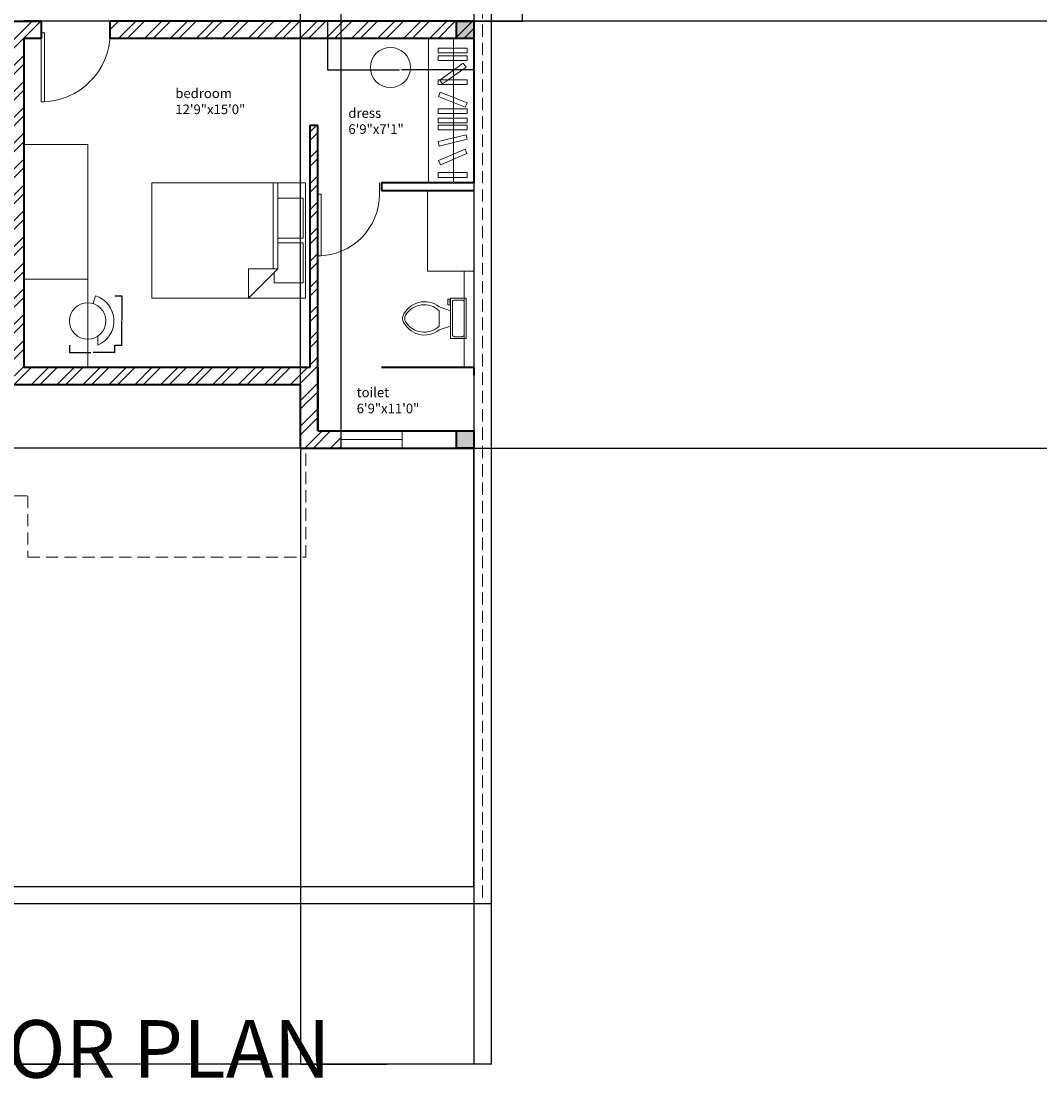
# Model space of a CAD drawing. Units: inches. Extents: x 19613 to 21413, y 12082 to 13202.
# Tile 2 of 9: x 19983 to 20513, y 12084 to 12634. Entities that reach past the tile are written whole.
import ezdxf

# ---------------------------------------------------------------- set-up
doc = ezdxf.new("R2010")
doc.units = ezdxf.units.IN
doc.linetypes.add('HIDDEN', pattern=[9.525, 6.35, -3.175])
for name, color, linetype, lineweight in [('A-ANNO-DIMS', 2, 'Continuous', 18), ('A-ANNO-TEXT', 7, 'Continuous', 30), ('A-AREA-IDEN', 7, 'Continuous', 18), ('A-COLS', 7, 'Continuous', 40), ('A-COLS-PATT', 6, 'Continuous', 13), ('A-DOOR', 3, 'Continuous', 18), ('A-FLOR-CASE', 9, 'Continuous', 18), ('A-FLOR-FIXT', 9, 'Continuous', 18), ('A-FLOR-HIDN', 8, 'HIDDEN', 13), ('A-FURN', 8, 'Continuous', 18), ('A-GLAZ', 4, 'Continuous', 18), ('A-WALL', 7, 'Continuous', 35), ('A-WALL-PATT', 252, 'Continuous', 13), ('C-PROP', 7, 'Continuous', 25), ('C-PROP-HIDN', 8, 'HIDDEN', 13)]:
    doc.layers.add(name, color=color, linetype=linetype, lineweight=lineweight)
doc.styles.get("Standard").update_dxf_attribs({"font": 'arial.ttf'})
doc.dimstyles.get("Standard").update_dxf_attribs({"dimtxt": 0.18, "dimasz": 0.18, "dimexe": 0.18, "dimexo": 0.0625, "dimgap": 0.09, "dimtad": 0, "dimtih": 1, "dimtoh": 1, "dimdec": 4, "dimzin": 0, "dimdsep": 46, "dimtxsty": 'Standard', "dimcen": 0.09, "dimadec": 0, "dimazin": 0, "dimtfac": 1, "dimtdec": 4, "dimtofl": 0, "dimtmove": 0, "dimatfit": 3, "dimfxl": 1, "dimtolj": 1, "dimtzin": 0, "dimarcsym": 0})

# ---------------------------------------------------------------- blocks, each defined once
blk = doc.blocks.new('Bed - Queen')
for p, q in [((0, -80.00003), (0, 0)), ((0, 0), (59.99999, 0)), ((59.99999, 0), (59.99999, -80.00003)), ((7.99999, -1.2), (28.79998, -1.2)), ((7.99999, -14.4), (7.99999, -1.2)), ((28.79998, -1.2), (28.79998, -14.4)), ((31.19999, -1.2), (51.99999, -1.2)), ((31.19999, -14.4), (31.19999, -1.2)), ((51.99999, -1.2), (51.99999, -16.4)), ((0, -14.4), (44.8, -14.4)), ((59.99999, -29.6), (44.8, -14.4)), ((44.8, -14.4), (44.8, -29.6)), ((51.99999, -16.4), (46.79936, -16.4)), ((44.8, -16.8), (0, -16.8)), ((44.8, -29.6), (59.99999, -29.6)), ((59.99999, -80.00003), (0, -80.00003))]:
    blk.add_line(p, q)
blk = doc.blocks.new('*U15')
for p, q in [((0, 0), (0, 6)), ((36, 0), (36, 6))]:
    blk.add_line(p, q)
blk.add_lwpolyline([(0, 0), (0, -36), (1.75, -36), (1.75, 0)], close=True)
blk.add_arc((0, 0), 36, 270, 0)
blk = doc.blocks.new('*U16')
for p, q in [((0, 0), (0, 6)), ((32, 0), (32, 6))]:
    blk.add_line(p, q)
blk.add_lwpolyline([(0, 0), (0, -32), (1.75, -32), (1.75, 0)], close=True)
blk.add_arc((0, 0), 32, 270, 0)
blk = doc.blocks.new('Toilet - top')
for p, q in [((9.5, -6), (9.5, -2)), ((-10, -8.5), (-8, -8.5)), ((-10, -9.5), (-10, -8.5)), ((-7, -9.5), (-10, -9.5)), ((-8, -8.5), (-8, -8)), ((-7, -8), (-7, -9.5)), ((-4, -8), (-6, -14)), ((4, -8), (6, -14)), ((4, -14), (-4, -14))]:
    blk.add_line(p, q)
blk.add_lwpolyline([(10.5, -8), (10.5, 0), (-10.5, 0), (-10.5, -8)], close=True)
for points in [[(-9.5, -2), (-9.5, -6)], [(8.5, -1), (-8.5, -1)], [(-8.5, -7), (8.5, -7)]]:
    blk.add_lwpolyline(points)
for centre, radius, start, end in [((-8.62, -1.88), 0.884, 81.8699, 188.1301), ((8.62, -1.88), 0.884, 351.8699, 98.1301), ((-8.62, -6.12), 0.884, 171.8699, 278.1301), ((8.62, -6.12), 0.884, 261.8699, 8.1301), ((3.52, -21.58), 12.17, 141.4691, 247.9714), ((4.2, -21.82), 11.33, 136.3677, 238.9468), ((-3.52, -21.58), 12.17, 292.0284, 38.5307), ((-4.2, -21.82), 11.33, 301.053, 43.6321), ((0, -27.88), 4, 245.7318, 294.2682), ((0, -29), 4, 254.8605, 285.1395)]:
    blk.add_arc(centre, radius, start, end)
blk = doc.blocks.new('COL-9x9')
for p, q in [((0, 9), (9, 9)), ((0, 0), (0, 9)), ((9, 9), (9, 0)), ((9, 0), (0, 0))]:
    blk.add_line(p, q)
blk = doc.blocks.new('CLOSET-STRAIGHT-RAIL')
for p, q in [((0, 75), (0, 0)), ((12.99, 75), (12.99, 0))]:
    blk.add_line(p, q)
for points in [[(5.04, 69.91), (20.08, 69.91), (20.08, 67.47), (5.04, 67.47)], [(5.04, 65.98), (20.08, 65.98), (20.08, 63.54), (5.04, 63.54)], [(5.8, 53.4), (18.07, 62.1), (19.48, 60.12), (7.21, 51.41)], [(5.04, 53.51), (20.08, 53.51), (20.08, 51.08), (5.04, 51.08)], [(6.02, 47.16), (20, 41.61), (19.1, 39.35), (5.12, 44.9)], [(5.04, 38.4), (20.08, 38.4), (20.08, 35.96), (5.04, 35.96)], [(5.04, 33.62), (20.08, 33.62), (20.08, 31.19), (5.04, 31.19)], [(5.04, 29.93), (20.08, 29.93), (20.08, 27.49), (5.04, 27.49)], [(4.97, 21.36), (19.58, 24.94), (20.16, 22.57), (5.55, 18.99)], [(5.22, 11.51), (19.01, 17.5), (19.98, 15.27), (6.19, 9.28)], [(5.04, 5.23), (20.08, 5.23), (20.08, 2.79), (5.04, 2.79)]]:
    blk.add_lwpolyline(points, close=True)
blk = doc.blocks.new('WINDOW-BATH')
for p, q in [((0, 9), (0, 0)), ((31.63, 9), (31.63, 0)), ((0, 4.5), (31.63, 4.5))]:
    blk.add_line(p, q)
blk = doc.blocks.new('DESK-CHAIR-ROUND-LARGE')
for p, q in [((13.49, 25.67), (12.27, 21.68)), ((14.77, 4.71), (14.81, 0))]:
    blk.add_line(p, q)
blk.add_circle((9.49, 12.6), 9.49)
blk.add_circle((9.49, 12.6), 9.49)
blk.add_arc((9.49, 12.6), 13.67, 292.8714, 73.0076)
blk = doc.blocks.new('BEDROOM-DESK-WIDE')
for p, q in [((33.29, 115.88), (0, 115.88)), ((33.29, 0), (33.29, 115.88)), ((33.29, 45.86), (0, 45.86)), ((0, 0), (0, 0)), ((0, 0), (33.29, 0))]:
    blk.add_line(p, q)
blk = doc.blocks.new('*D71')
at = {"layer": 'A-ANNO-DIMS', "color": 0, "lineweight": -2, "transparency": 16777216}
for p, q in [((20032, 12491.47), (20035.96, 12491.47)), ((20035.78, 12491.29), (20035.78, 12478.81)), ((20035.78, 12465.98), (20035.78, 12478.45)), ((20032, 12465.8), (20035.96, 12465.8))]:
    blk.add_line(p, q, dxfattribs=at)
at = {"layer": 'A-ANNO-DIMS', "color": 0, "transparency": 16777216}
for points in [[(20035.75, 12491.29), (20035.81, 12491.29), (20035.78, 12491.47)], [(20035.75, 12465.98), (20035.81, 12465.98), (20035.78, 12465.8)]]:
    blk.add_solid(points, dxfattribs=at)
at = {"layer": 'Defpoints', "color": 0, "transparency": 16777216}
for p in [(20031.93, 12491.47), (20035.78, 12491.47), (20031.93, 12465.8)]:
    blk.add_point(p, dxfattribs=at)
at = {"layer": 'A-ANNO-DIMS', "color": 0, "transparency": 16777216, "insert": (20035.78, 12478.63), "char_height": 0.18, "attachment_point": 5}
blk.add_mtext('\\A1;CHAIR 26 TYP.', dxfattribs=at)
blk = doc.blocks.new('*D72')
at = {"layer": 'A-ANNO-DIMS', "color": 0, "lineweight": -2, "transparency": 16777216}
for p, q in [((20008.49, 12465.73), (20008.49, 12461.76)), ((20031.93, 12465.73), (20031.93, 12461.76)), ((20008.67, 12461.94), (20019.68, 12461.94)), ((20031.75, 12461.94), (20020.74, 12461.94))]:
    blk.add_line(p, q, dxfattribs=at)
at = {"layer": 'A-ANNO-DIMS', "color": 0, "transparency": 16777216}
for points in [[(20008.67, 12461.97), (20008.67, 12461.91), (20008.49, 12461.94)], [(20031.75, 12461.97), (20031.75, 12461.91), (20031.93, 12461.94)]]:
    blk.add_solid(points, dxfattribs=at)
at = {"layer": 'Defpoints', "color": 0, "transparency": 16777216}
for p in [(20008.49, 12465.8), (20031.93, 12465.8), (20031.93, 12461.94)]:
    blk.add_point(p, dxfattribs=at)
at = {"layer": 'A-ANNO-DIMS', "color": 0, "transparency": 16777216, "insert": (20020.21, 12461.94), "char_height": 0.18, "attachment_point": 5}
blk.add_mtext('\\A1;23 TYP.', dxfattribs=at)
blk = doc.blocks.new('*D77')
at = {"layer": 'A-ANNO-DIMS', "color": 0, "lineweight": -2, "transparency": 16777216}
for p, q in [((20218.76, 12803.28), (20244.22, 12803.28)), ((20244.04, 12803.1), (20244.04, 12718.96)), ((20244.04, 12634.46), (20244.04, 12718.6)), ((20218.76, 12634.28), (20244.22, 12634.28))]:
    blk.add_line(p, q, dxfattribs=at)
at = {"layer": 'A-ANNO-DIMS', "color": 0, "transparency": 16777216}
for points in [[(20244.01, 12803.1), (20244.07, 12803.1), (20244.04, 12803.28)], [(20244.01, 12634.46), (20244.07, 12634.46), (20244.04, 12634.28)]]:
    blk.add_solid(points, dxfattribs=at)
at = {"layer": 'Defpoints', "color": 0, "transparency": 16777216}
for p in [(20218.69, 12803.28), (20244.04, 12803.28), (20218.69, 12634.28)]:
    blk.add_point(p, dxfattribs=at)
at = {"layer": 'A-ANNO-DIMS', "color": 0, "transparency": 16777216, "insert": (20244.04, 12718.78), "char_height": 0.18, "attachment_point": 5}
blk.add_mtext('\\A1;STAIR 169 TYP.', dxfattribs=at)
blk = doc.blocks.new('*D78')
at = {"layer": 'A-ANNO-DIMS', "color": 0, "lineweight": -2, "transparency": 16777216}
for p, q in [((20142.69, 12634.22), (20142.69, 12608.75)), ((20218.69, 12634.22), (20218.69, 12608.75)), ((20142.87, 12608.93), (20180.17, 12608.93)), ((20218.51, 12608.93), (20181.22, 12608.93))]:
    blk.add_line(p, q, dxfattribs=at)
at = {"layer": 'A-ANNO-DIMS', "color": 0, "transparency": 16777216}
for points in [[(20142.87, 12608.96), (20142.87, 12608.9), (20142.69, 12608.93)], [(20218.51, 12608.96), (20218.51, 12608.9), (20218.69, 12608.93)]]:
    blk.add_solid(points, dxfattribs=at)
at = {"layer": 'Defpoints', "color": 0, "transparency": 16777216}
for p in [(20142.69, 12634.28), (20218.69, 12634.28), (20218.69, 12608.93)]:
    blk.add_point(p, dxfattribs=at)
at = {"layer": 'A-ANNO-DIMS', "color": 0, "transparency": 16777216, "insert": (20180.69, 12608.93), "char_height": 0.18, "attachment_point": 5}
blk.add_mtext('\\A1;76 TYP.', dxfattribs=at)
blk = doc.blocks.new('*D83')
at = {"layer": 'A-ANNO-DIMS', "color": 0, "lineweight": -2, "transparency": 16777216}
for p, q in [((19696.69, 12175.22), (19696.69, 12091.85)), ((20227.69, 12175.22), (20227.69, 12091.85)), ((19696.87, 12092.03), (19961.92, 12092.03)), ((20227.51, 12092.03), (19962.47, 12092.03))]:
    blk.add_line(p, q, dxfattribs=at)
at = {"layer": 'A-ANNO-DIMS', "color": 0, "transparency": 16777216}
for points in [[(19696.87, 12092.06), (19696.87, 12092), (19696.69, 12092.03)], [(20227.51, 12092.06), (20227.51, 12092), (20227.69, 12092.03)]]:
    blk.add_solid(points, dxfattribs=at)
at = {"layer": 'Defpoints', "color": 0, "transparency": 16777216}
for p in [(19696.69, 12175.28), (20227.69, 12175.28), (20227.69, 12092.03)]:
    blk.add_point(p, dxfattribs=at)
at = {"layer": 'A-ANNO-DIMS', "color": 0, "transparency": 16777216, "insert": (19962.19, 12092.03), "char_height": 0.18, "attachment_point": 5}
blk.add_mtext('\\A1;531', dxfattribs=at)
blk = doc.blocks.new('*D87')
at = {"layer": 'A-ANNO-DIMS', "color": 0, "lineweight": -2, "transparency": 16777216}
for p, q in [((20218.76, 12982.28), (21412.86, 12982.28)), ((21412.68, 12982.1), (21412.68, 12697.46)), ((21412.68, 12412.46), (21412.68, 12697.1)), ((20218.76, 12412.28), (21412.86, 12412.28))]:
    blk.add_line(p, q, dxfattribs=at)
at = {"layer": 'A-ANNO-DIMS', "color": 0, "transparency": 16777216}
for points in [[(21412.65, 12982.1), (21412.71, 12982.1), (21412.68, 12982.28)], [(21412.65, 12412.46), (21412.71, 12412.46), (21412.68, 12412.28)]]:
    blk.add_solid(points, dxfattribs=at)
at = {"layer": 'Defpoints', "color": 0, "transparency": 16777216}
for p in [(20218.69, 12982.28), (21412.68, 12982.28), (20218.69, 12412.28)]:
    blk.add_point(p, dxfattribs=at)
at = {"layer": 'A-ANNO-DIMS', "color": 0, "transparency": 16777216, "insert": (21412.68, 12697.28), "char_height": 0.18, "attachment_point": 5}
blk.add_mtext('\\A1;570', dxfattribs=at)
blk = doc.blocks.new('*D89')
at = {"layer": 'A-ANNO-DIMS', "color": 0, "lineweight": -2, "transparency": 16777216}
for p, q in [((20807.37, 12808.28), (19613.26, 12808.28)), ((19613.44, 12808.1), (19613.44, 12721.46)), ((19613.44, 12634.46), (19613.44, 12721.1)), ((20807.37, 12634.28), (19613.26, 12634.28))]:
    blk.add_line(p, q, dxfattribs=at)
at = {"layer": 'A-ANNO-DIMS', "color": 0, "transparency": 16777216}
for points in [[(19613.41, 12808.1), (19613.47, 12808.1), (19613.44, 12808.28)], [(19613.41, 12634.46), (19613.47, 12634.46), (19613.44, 12634.28)]]:
    blk.add_solid(points, dxfattribs=at)
at = {"layer": 'Defpoints', "color": 0, "transparency": 16777216}
for p in [(19613.44, 12808.28), (20807.43, 12808.28), (20807.43, 12634.28)]:
    blk.add_point(p, dxfattribs=at)
at = {"layer": 'A-ANNO-DIMS', "color": 0, "transparency": 16777216, "insert": (19613.44, 12721.28), "char_height": 0.18, "attachment_point": 5}
blk.add_mtext('\\A1;174', dxfattribs=at)
blk = doc.blocks.new('*D92')
at = {"layer": 'A-ANNO-DIMS', "color": 0, "lineweight": -2, "transparency": 16777216}
for p, q in [((19903.69, 12445.22), (19903.69, 12091.85)), ((20128.69, 12445.22), (20128.69, 12091.85)), ((19903.87, 12092.03), (20015.9, 12092.03)), ((20128.51, 12092.03), (20016.48, 12092.03))]:
    blk.add_line(p, q, dxfattribs=at)
at = {"layer": 'A-ANNO-DIMS', "color": 0, "transparency": 16777216}
for points in [[(19903.87, 12092.06), (19903.87, 12092), (19903.69, 12092.03)], [(20128.51, 12092.06), (20128.51, 12092), (20128.69, 12092.03)]]:
    blk.add_solid(points, dxfattribs=at)
at = {"layer": 'Defpoints', "color": 0, "transparency": 16777216}
for p in [(19903.69, 12445.28), (20128.69, 12445.28), (20128.69, 12092.03)]:
    blk.add_point(p, dxfattribs=at)
at = {"layer": 'A-ANNO-DIMS', "color": 0, "transparency": 16777216, "insert": (20016.19, 12092.03), "char_height": 0.18, "attachment_point": 5}
blk.add_mtext('\\A1;225', dxfattribs=at)
blk = doc.blocks.new('*D93')
at = {"layer": 'A-ANNO-DIMS', "color": 0, "lineweight": -2, "transparency": 16777216}
for p, q in [((20128.69, 12412.22), (20128.69, 12091.85)), ((20218.69, 12412.22), (20218.69, 12091.85)), ((20128.87, 12092.03), (20173.48, 12092.03)), ((20218.51, 12092.03), (20173.91, 12092.03))]:
    blk.add_line(p, q, dxfattribs=at)
at = {"layer": 'A-ANNO-DIMS', "color": 0, "transparency": 16777216}
for points in [[(20128.87, 12092.06), (20128.87, 12092), (20128.69, 12092.03)], [(20218.51, 12092.06), (20218.51, 12092), (20218.69, 12092.03)]]:
    blk.add_solid(points, dxfattribs=at)
at = {"layer": 'Defpoints', "color": 0, "transparency": 16777216}
for p in [(20128.69, 12412.28), (20218.69, 12412.28), (20218.69, 12092.03)]:
    blk.add_point(p, dxfattribs=at)
at = {"layer": 'A-ANNO-DIMS', "color": 0, "transparency": 16777216, "insert": (20173.69, 12092.03), "char_height": 0.18, "attachment_point": 5}
blk.add_mtext('\\A1;90', dxfattribs=at)
blk = doc.blocks.new('*D97')
at = {"layer": 'A-ANNO-DIMS', "color": 0, "lineweight": -2, "transparency": 16777216}
for p, q in [((20128.63, 12445.28), (19613.26, 12445.28)), ((19613.44, 12445.1), (19613.44, 12428.96)), ((19613.44, 12412.46), (19613.44, 12428.6)), ((20128.63, 12412.28), (19613.26, 12412.28))]:
    blk.add_line(p, q, dxfattribs=at)
at = {"layer": 'A-ANNO-DIMS', "color": 0, "transparency": 16777216}
for points in [[(19613.41, 12445.1), (19613.47, 12445.1), (19613.44, 12445.28)], [(19613.41, 12412.46), (19613.47, 12412.46), (19613.44, 12412.28)]]:
    blk.add_solid(points, dxfattribs=at)
at = {"layer": 'Defpoints', "color": 0, "transparency": 16777216}
for p in [(19613.44, 12445.28), (20128.69, 12445.28), (20128.69, 12412.28)]:
    blk.add_point(p, dxfattribs=at)
at = {"layer": 'A-ANNO-DIMS', "color": 0, "transparency": 16777216, "insert": (19613.44, 12428.78), "char_height": 0.18, "attachment_point": 5}
blk.add_mtext('\\A1;33', dxfattribs=at)
blk = doc.blocks.new('*D107')
at = {"layer": 'A-ANNO-DIMS', "color": 0, "lineweight": -2, "transparency": 16777216}
for p, q in [((20128.69, 12412.34), (20128.69, 13201.71)), ((20128.87, 13201.53), (20138.81, 13201.53)), ((20149.67, 13201.53), (20139.74, 13201.53)), ((20149.85, 12412.34), (20149.85, 13201.71))]:
    blk.add_line(p, q, dxfattribs=at)
at = {"layer": 'A-ANNO-DIMS', "color": 0, "transparency": 16777216}
for points in [[(20128.87, 13201.56), (20128.87, 13201.5), (20128.69, 13201.53)], [(20149.67, 13201.56), (20149.67, 13201.5), (20149.85, 13201.53)]]:
    blk.add_solid(points, dxfattribs=at)
at = {"layer": 'Defpoints', "color": 0, "transparency": 16777216}
for p in [(20149.85, 13201.53), (20128.69, 12412.28), (20149.85, 12412.28)]:
    blk.add_point(p, dxfattribs=at)
at = {"layer": 'A-ANNO-DIMS', "color": 0, "transparency": 16777216, "insert": (20139.27, 13201.53), "char_height": 0.18, "attachment_point": 5}
blk.add_mtext('\\A1;21.154', dxfattribs=at)

msp = doc.modelspace()

# ---------------------------------------------------------------- hatches: boundary and pattern name
at = {"layer": 'A-COLS-PATT'}
h = msp.add_hatch(color=256, dxfattribs=at)
h.dxf.hatch_style = 1
h.paths.add_polyline_path([(19701.1937, 13118.279), (19696.6937, 13118.279), (19696.6937, 13113.779), (19701.1937, 13113.779)])
h.paths.add_polyline_path([(19714.6694, 12982.279), (19705.6937, 12982.279), (19705.6937, 12973.279), (19714.6694, 12973.279)])
h.paths.add_polyline_path([(19827.1183, 12982.279), (19818.1183, 12982.279), (19818.1183, 12973.279), (19827.1183, 12973.279)])
h.paths.add_polyline_path([(19982.6937, 12982.279), (19973.6937, 12982.279), (19973.6937, 12973.279), (19982.6937, 12973.279)])
h.paths.add_polyline_path([(19982.6937, 12817.279), (19973.6937, 12817.279), (19973.6937, 12808.279), (19982.6937, 12808.279)])
h.paths.add_polyline_path([(19795.361, 12817.279), (19786.361, 12817.279), (19786.361, 12808.279), (19795.361, 12808.279)])
h.paths.add_polyline_path([(19705.6937, 12817.279), (19702.0819, 12817.279), (19702.0819, 12808.279), (19705.6937, 12808.279)])
h.paths.add_polyline_path([(19711.0819, 12817.279), (19705.6937, 12817.279), (19705.6937, 12808.279), (19711.0819, 12808.279)])
h.paths.add_polyline_path([(19714.6136, 12634.279), (19705.6937, 12634.279), (19705.6937, 12625.279), (19714.6136, 12625.279)])
h.paths.add_polyline_path([(19705.6937, 12485.8897), (19701.1937, 12485.8897), (19701.1937, 12476.8897), (19705.6937, 12476.8897)])
h.paths.add_polyline_path([(19709.3479, 12485.8897), (19705.6937, 12485.8897), (19705.6937, 12476.8897), (19709.3479, 12476.8897)])
h.paths.add_polyline_path([(19701.1937, 12485.8897), (19700.3479, 12485.8897), (19700.3479, 12476.8897), (19701.1937, 12476.8897)])
h.paths.add_polyline_path([(20218.6937, 12421.279), (20209.6937, 12421.279), (20209.6937, 12412.279), (20218.6937, 12412.279)])
h.paths.add_polyline_path([(20218.6937, 12634.279), (20209.6937, 12634.279), (20209.6937, 12625.279), (20218.6937, 12625.279)])
h.paths.add_polyline_path([(20218.6937, 12808.279), (20209.6937, 12808.279), (20209.6937, 12803.279), (20218.6937, 12803.279)])
h.paths.add_polyline_path([(20218.6937, 12810.1878), (20209.6937, 12810.1878), (20209.6937, 12808.279), (20218.6937, 12808.279)])
h.paths.add_polyline_path([(20218.6937, 12803.279), (20209.6937, 12803.279), (20209.6937, 12801.1878), (20218.6937, 12801.1878)])
h.paths.add_polyline_path([(20218.6937, 12982.279), (20209.6937, 12982.279), (20209.6937, 12973.279), (20218.6937, 12973.279)])
h.paths.add_polyline_path([(20100.1214, 12982.279), (20080.8386, 12982.279), (20080.8386, 12973.279), (20091.6937, 12973.279), (20100.1214, 12973.279), (20100.1214, 12976.279)])
h.paths.add_polyline_path([(19851.5503, 12631.279), (19851.5503, 12634.279), (19828.8814, 12634.279), (19828.8814, 12625.279), (19851.5503, 12625.279)])
at = {"layer": 'A-WALL-PATT'}
h = msp.add_hatch(dxfattribs=at)
h.set_pattern_fill('ANSI32', color=256)
h.paths.add_polyline_path([(20223.1937, 13118.279), (20218.6937, 13118.279), (19701.1937, 13118.279), (19701.1937, 13113.779), (20223.1937, 13113.779)])
h.paths.add_polyline_path([(19849.7315, 12982.279), (19799.9854, 12982.279), (19799.9854, 12973.279), (19849.7315, 12973.279)])
h.paths.add_polyline_path([(19755.5378, 12982.279), (19705.6937, 12982.279), (19705.6937, 12973.279), (19755.5378, 12973.279)])
h.paths.add_polyline_path([(20000.1054, 12982.279), (19950.0534, 12982.279), (19950.0534, 12974.1171), (19950.0534, 12973.279), (20000.1054, 12973.279)])
h.paths.add_polyline_path([(20049.4797, 12982.279), (20030.7476, 12982.279), (20030.7476, 12973.279), (20049.4797, 12973.279)])
h.paths.add_polyline_path([(20100.1214, 12982.279), (20080.8386, 12982.279), (20080.8386, 12973.279), (20100.1214, 12973.279), (20100.1214, 12976.279)])
h.paths.add_polyline_path([(20218.6937, 12982.279), (20167.6937, 12982.279), (20140.1214, 12982.279), (20140.1214, 12976.279, -0.01769781), (20140.0212, 12973.45), (20167.6937, 12973.279), (20176.6937, 12973.279), (20218.6937, 12973.279)])
h.paths.add_polyline_path([(19851.5503, 12814.279), (19851.5503, 12817.279), (19793.6937, 12817.279), (19789.6937, 12817.279), (19705.6937, 12817.279), (19705.6937, 12808.279), (19851.5503, 12808.279)])
h.paths.add_polyline_path([(19982.6937, 12973.279), (19973.6937, 12973.279), (19973.6937, 12817.279), (19887.5503, 12817.279), (19887.5503, 12808.279), (19973.6937, 12808.279), (19982.6937, 12808.279)])
h.paths.add_polyline_path([(20058.6937, 12850.5529), (19982.6937, 12850.5529), (19982.6937, 12846.5529), (20058.6937, 12846.5529)])
h.paths.add_polyline_path([(20095.6937, 12973.279), (20091.6937, 12973.279), (20091.6937, 12850.5529), (20087.6937, 12850.5529), (20087.6937, 12846.5529), (20095.6937, 12846.5529)])
h.paths.add_polyline_path([(20218.6937, 12808.279), (20140.8605, 12808.279), (20126.9413, 12808.279), (20126.9413, 12803.279), (20140.8605, 12803.279), (20218.6937, 12803.279)])
h.paths.add_polyline_path([(19738.3931, 12634.279), (19705.6937, 12634.279), (19705.6937, 12625.279), (19738.3931, 12625.279)])
h.paths.add_polyline_path([(19912.6937, 12634.279), (19903.6937, 12634.279), (19891.5503, 12634.279), (19891.5503, 12625.279), (19903.6937, 12625.279), (19903.6937, 12445.279), (19975.6937, 12445.279), (20128.6937, 12445.279), (20128.6937, 12412.279), (20149.8479, 12412.279), (20149.8479, 12421.279), (20137.6937, 12421.279), (20137.6937, 12454.279), (20137.6937, 12580.2801), (20133.6937, 12580.2801), (20133.6937, 12454.279), (19984.6937, 12454.279), (19984.6937, 12625.279), (19993.6937, 12625.279), (19993.6937, 12634.279), (19984.6937, 12634.279), (19975.6937, 12634.279), (19975.6937, 12454.279), (19912.6937, 12454.279)])
h.paths.add_polyline_path([(20218.6937, 12634.279), (20137.6937, 12634.279), (20029.6937, 12634.279), (20029.6937, 12625.279), (20137.6937, 12625.279), (20218.6937, 12625.279)])
h.paths.add_polyline_path([(21014.4339, 12634.279), (21005.4339, 12634.279), (20993.2905, 12634.279), (20993.2905, 12625.279), (21005.4339, 12625.279), (21005.4339, 12445.279), (21077.4339, 12445.279), (21230.4339, 12445.279), (21230.4339, 12412.279), (21251.5881, 12412.279), (21251.5881, 12421.279), (21239.4339, 12421.279), (21239.4339, 12454.279), (21239.4339, 12580.2801), (21235.4339, 12580.2801), (21235.4339, 12454.279), (21086.4339, 12454.279), (21086.4339, 12625.279), (21095.4339, 12625.279), (21095.4339, 12634.279), (21086.4339, 12634.279), (21077.4339, 12634.279), (21077.4339, 12454.279), (21014.4339, 12454.279)])
h.paths.add_polyline_path([(20840.1333, 12634.279), (20807.4339, 12634.279), (20807.4339, 12625.279), (20840.1333, 12625.279)])
h.paths.add_polyline_path([(20953.2905, 12631.279), (20953.2905, 12634.279), (20930.6216, 12634.279), (20930.6216, 12625.279), (20953.2905, 12625.279)])
h.paths.add_polyline_path([(21320.4339, 12634.279), (21239.4339, 12634.279), (21131.4339, 12634.279), (21131.4339, 12625.279), (21239.4339, 12625.279), (21320.4339, 12625.279)])
h.paths.add_polyline_path([(21084.4339, 12973.279), (21075.4339, 12973.279), (21075.4339, 12817.279), (20989.2905, 12817.279), (20989.2905, 12808.279), (21075.4339, 12808.279), (21084.4339, 12808.279)])
h.paths.add_polyline_path([(21142.1261, 12863.2893), (21084.4339, 12863.2893), (21084.4339, 12846.5529), (21142.1261, 12846.5529)])
h.paths.add_polyline_path([(21320.4339, 12808.279), (21242.6007, 12808.279), (21228.6815, 12808.279), (21228.6815, 12803.279), (21242.6007, 12803.279), (21320.4339, 12803.279)])
h.paths.add_polyline_path([(20857.278, 12982.279), (20807.4339, 12982.279), (20807.4339, 12973.279), (20857.278, 12973.279)])
h.paths.add_polyline_path([(20951.4717, 12982.279), (20901.7255, 12982.279), (20901.7255, 12973.279), (20951.4717, 12973.279)])
h.paths.add_polyline_path([(21101.8455, 12982.279), (21051.7936, 12982.279), (21051.7936, 12974.1171), (21051.7936, 12973.279), (21101.8455, 12973.279)])
h.paths.add_polyline_path([(21151.2199, 12982.279), (21132.4878, 12982.279), (21132.4878, 12973.279), (21151.2199, 12973.279)])
h.paths.add_polyline_path([(21201.8616, 12982.279), (21182.5788, 12982.279), (21182.5788, 12973.279), (21193.4339, 12973.279), (21201.8616, 12973.279), (21201.8616, 12976.279)])
h.paths.add_polyline_path([(21320.4339, 12982.279), (21269.4339, 12982.279), (21241.8616, 12982.279), (21241.8616, 12976.279, -0.01769781), (21241.7614, 12973.45), (21269.4339, 12973.279), (21278.4339, 12973.279), (21320.4339, 12973.279)])
h.paths.add_polyline_path([(20953.2905, 12817.279), (20895.4339, 12817.279), (20891.4339, 12817.279), (20807.4339, 12817.279), (20807.4339, 12808.279), (20953.2905, 12808.279)])
h.paths.add_polyline_path([(21197.4339, 12973.279), (21193.4339, 12973.279), (21193.4339, 12850.5529), (21197.4339, 12850.5529)])
h.paths.add_polyline_path([(21320.4339, 12550.279), (21272.5278, 12550.279), (21272.5278, 12546.279), (21320.4339, 12546.279)])
h.paths.add_polyline_path([(21320.4339, 12421.279), (21283.2222, 12421.279), (21283.2222, 12412.279), (21320.4339, 12412.279)])

# ---------------------------------------------------------------- linework, layer by layer
at = {"layer": 'A-FLOR-FIXT'}
for p, q in [((20194.7407, 12546.279), (20194.7407, 12504.2908)), ((20194.7407, 12504.2908), (20218.6937, 12504.2908)), ((20218.6937, 12504.2908), (20213.6937, 12504.2908)), ((20213.6937, 12504.2908), (20213.6937, 12454.279))]:
    msp.add_line(p, q, dxfattribs=at)
at = {"layer": 'A-FLOR-HIDN'}
for p, q in [((20131.3568, 12355.488), (20131.3568, 12412.279)), ((19903.6937, 12387.4793), (19986.7757, 12387.4793)), ((19986.7757, 12387.4793), (19986.7757, 12355.488)), ((19986.7757, 12355.488), (20131.3568, 12355.488))]:
    msp.add_line(p, q, dxfattribs=at)
at = {"layer": 'A-FURN'}
msp.add_circle((20175.3687, 12610.1834), 10.4264, dxfattribs=at)
at = {"layer": 'A-WALL'}
for p, q in [((19975.6937, 12634.279), (19984.6937, 12634.279)), ((19984.6937, 12634.279), (19993.6937, 12634.279)), ((19993.6937, 12634.279), (19984.6937, 12634.279)), ((19993.6937, 12634.279), (19993.6937, 12625.279)), ((20137.6937, 12634.279), (20029.6937, 12634.279)), ((20029.6937, 12625.279), (20029.6937, 12634.279)), ((20218.6937, 12634.279), (20137.6937, 12634.279)), ((20218.6937, 12634.279), (20218.6937, 12550.279)), ((19984.6937, 12625.279), (19984.6937, 12454.279)), ((19993.6937, 12625.279), (19984.6937, 12625.279)), ((20137.6937, 12625.279), (20029.6937, 12625.279)), ((20218.6937, 12625.279), (20137.6937, 12625.279)), ((20133.6937, 12454.279), (20133.6937, 12580.2801)), ((20133.6937, 12580.2801), (20137.6937, 12580.2801)), ((20137.6937, 12454.279), (20137.6937, 12580.2801)), ((20218.6937, 12550.279), (20170.7877, 12550.279)), ((20170.7877, 12550.279), (20170.7877, 12546.279)), ((20170.7877, 12546.279), (20218.6937, 12546.279)), ((19984.6937, 12454.279), (20133.6937, 12454.279)), ((20137.6937, 12454.279), (20137.6937, 12421.279)), ((20137.6937, 12421.279), (20137.6937, 12454.279)), ((20137.6937, 12421.279), (20137.6937, 12454.279)), ((20170.7877, 12454.279), (20218.6937, 12454.279)), ((20218.6937, 12454.279), (20218.6937, 12450.279)), ((19975.6937, 12445.279), (20128.6937, 12445.279)), ((20128.6937, 12412.279), (20128.6937, 12445.279)), ((20137.6937, 12421.279), (20218.6937, 12421.279)), ((20128.6937, 12412.279), (20218.6937, 12412.279))]:
    msp.add_line(p, q, dxfattribs=at)
at = {"layer": 'C-PROP'}
for p, q in [((20227.6937, 13118.279), (20227.6937, 12175.279)), ((20218.6937, 13109.279), (20218.6937, 12184.279)), ((20218.6937, 12184.279), (20218.6937, 12412.279)), ((19705.6937, 12184.279), (20218.6937, 12184.279)), ((20227.6937, 12175.279), (19696.6937, 12175.279))]:
    msp.add_line(p, q, dxfattribs=at)
at = {"layer": 'C-PROP-HIDN'}
msp.add_line((20223.1937, 13118.279), (20223.1937, 12175.279), dxfattribs=at)

# ---------------------------------------------------------------- block references
at = {"layer": 'A-COLS', "rotation": 180}
for p in [(20218.6941, 12634.279), (20218.6941, 12421.279)]:
    msp.add_blockref('COL-9x9', p, dxfattribs=at)
at = {"layer": 'A-DOOR'}
for name, p in [('*U15', (19993.6937, 12628.279)), ('*U16', (20137.6937, 12544.279))]:
    msp.add_blockref(name, p, dxfattribs=at)
at = {"layer": 'A-FLOR-CASE'}
msp.add_blockref('CLOSET-STRAIGHT-RAIL', (20195.197, 12550.279), dxfattribs=at)
at = {"layer": 'A-FLOR-FIXT', "rotation": 270}
msp.add_blockref('Toilet - top', (20214.6848, 12479.7213), dxfattribs=at)
at = {"layer": 'A-FURN'}
for name, p in [('BEDROOM-DESK-WIDE', (19984.694, 12454.279)), ('DESK-CHAIR-ROUND-LARGE', (20008.492, 12465.795))]:
    msp.add_blockref(name, p, dxfattribs=at)
at = {"layer": 'A-FURN', "rotation": 270.0000000000108}
msp.add_blockref('Bed - Queen', (20131.256, 12550.2322), dxfattribs=at)
at = {"layer": 'A-GLAZ'}
msp.add_blockref('WINDOW-BATH', (20149.848, 12412.279), dxfattribs=at)

# ---------------------------------------------------------------- texts
at = {"layer": 'A-ANNO-TEXT', "insert": (19719.9437, 12114.8481), "char_height": 30, "attachment_point": 1}
msp.add_mtext_dynamic_manual_height_columns('GROUND FLOOR PLAN', width=510.437427, gutter_width=12.5, heights=[0], dxfattribs=at)
at = {"layer": 'A-AREA-IDEN', "char_height": 5, "attachment_point": 1}
for s, insert in [('bedroom\\P12\'9"x15\'0"', (20063.5197, 12599.2649)), ('dress\\P6\'9"x7\'1"', (20153.5154, 12588.9924)), ('toilet\\P6\'9"x11\'0"', (20157.8239, 12443.7325))]:
    msp.add_mtext_dynamic_manual_height_columns(s, width=19.652904, gutter_width=12.5, heights=[0], dxfattribs=dict(at, insert=insert))

# ---------------------------------------------------------------- dimensions: what is measured, and where the dimension line sits
at = {"layer": 'A-ANNO-DIMS'}
for base, p1, p2, override, picture, middle in [((20149.8479, 13201.529), (20128.6937, 12412.279), (20149.8479, 12412.279), {"dimdec": 3, "dimlfac": 1, "dimrnd": 0, "dimzin": 0, "dimdsep": 46, "dimlunit": 2}, '*D107', (20139.2708, 13201.529)), ((20128.6937, 12092.029), (19903.6937, 12445.279), (20128.6937, 12445.279), {"dimdec": 0, "dimlfac": 1, "dimrnd": 0, "dimzin": 0, "dimdsep": 46, "dimlunit": 2}, '*D92', (20016.1937, 12092.029)), ((20218.6937, 12092.029), (20128.6937, 12412.279), (20218.6937, 12412.279), {"dimdec": 0, "dimlfac": 1, "dimrnd": 0, "dimzin": 0, "dimdsep": 46, "dimlunit": 2}, '*D93', (20173.6937, 12092.029)), ((20227.6937, 12092.029), (19696.6937, 12175.279), (20227.6937, 12175.279), {"dimdec": 0, "dimlfac": 1, "dimrnd": 0, "dimzin": 0, "dimdsep": 46, "dimlunit": 2}, '*D83', (19962.1937, 12092.029))]:
    dim = msp.add_linear_dim(base=base, p1=p1, p2=p2, dimstyle='Standard', override=override, dxfattribs=at)
    dim.commit()
    dim.dimension.update_dxf_attribs({"geometry": picture, "text_midpoint": middle})
for base, p1, p2, picture, middle in [((21412.6839, 12982.279), (20218.6937, 12412.279), (20218.6937, 12982.279), '*D87', (21412.6839, 12697.279)), ((19613.4437, 12808.279), (20807.4339, 12634.279), (20807.4339, 12808.279), '*D89', (19613.4437, 12721.279)), ((19613.4437, 12445.279), (20128.6937, 12412.279), (20128.6937, 12445.279), '*D97', (19613.4437, 12428.779))]:
    dim = msp.add_linear_dim(base=base, p1=p1, p2=p2, angle=90, dimstyle='Standard', override={"dimdec": 0, "dimlfac": 1, "dimrnd": 0, "dimzin": 0, "dimdsep": 46, "dimlunit": 2}, dxfattribs=at)
    dim.commit()
    dim.dimension.update_dxf_attribs({"geometry": picture, "text_midpoint": middle})
for base, p1, p2, text, picture, middle in [((20244.0437, 12803.279), (20218.6937, 12634.279), (20218.6937, 12803.279), 'STAIR <> TYP.', '*D77', (20244.0437, 12718.779)), ((20035.7848, 12491.4673), (20031.9339, 12465.7952), (20031.9339, 12491.4673), 'CHAIR <> TYP.', '*D71', (20035.7848, 12478.6313))]:
    dim = msp.add_linear_dim(base=base, p1=p1, p2=p2, angle=90, text=text, dimstyle='Standard', override={"dimdec": 0, "dimlfac": 1, "dimrnd": 0, "dimzin": 0, "dimdsep": 46, "dimlunit": 2}, dxfattribs=at)
    dim.commit()
    dim.dimension.update_dxf_attribs({"geometry": picture, "text_midpoint": middle})
for base, p1, p2, picture, middle in [((20218.6937, 12608.929), (20142.6937, 12634.279), (20218.6937, 12634.279), '*D78', (20180.6937, 12608.929)), ((20031.9339, 12461.9444), (20008.4924, 12465.7952), (20031.9339, 12465.7952), '*D72', (20020.2132, 12461.9444))]:
    dim = msp.add_linear_dim(base=base, p1=p1, p2=p2, text='<> TYP.', dimstyle='Standard', override={"dimdec": 0, "dimlfac": 1, "dimrnd": 0, "dimzin": 0, "dimdsep": 46, "dimlunit": 2}, dxfattribs=at)
    dim.commit()
    dim.dimension.update_dxf_attribs({"geometry": picture, "text_midpoint": middle})

doc.saveas('drawing.dxf')
